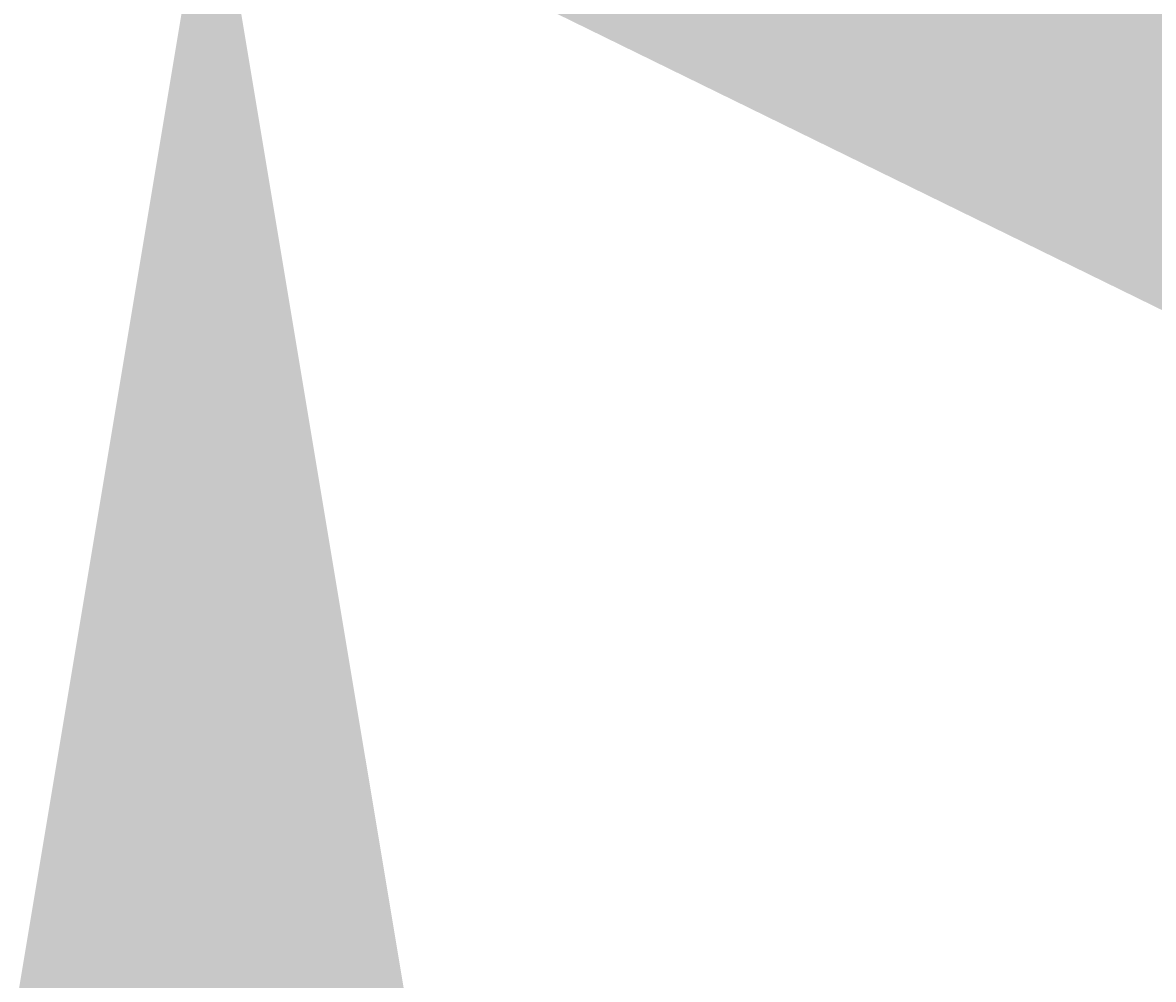
# Model space of a CAD drawing. Units: millimetres. Extents: x -22994 to 29398, y -19990 to 20176.
# Tile 5 of 135: x -44 to 2052, y -1986 to -212. Entities that reach past the tile are written whole.
import ezdxf

# ---------------------------------------------------------------- set-up
doc = ezdxf.new("R2010")
doc.units = ezdxf.units.MM
doc.header["$MEASUREMENT"] = 0
doc.layers.add('M-DIMS', color=2, linetype='Continuous', lineweight=18)
doc.styles.get("Standard").update_dxf_attribs({"font": 'arial.ttf'})
doc.dimstyles.get("Standard").update_dxf_attribs({"dimtxt": 0.18, "dimasz": 10000, "dimexe": 0.18, "dimexo": 0.0625, "dimgap": 0.09, "dimtad": 0, "dimtih": 1, "dimtoh": 1, "dimdec": 0, "dimzin": 0, "dimdsep": 46, "dimtxsty": 'Standard', "dimcen": 0.09, "dimadec": 0, "dimazin": 0, "dimtfac": 1, "dimtdec": 0, "dimtofl": 0, "dimtmove": 0, "dimatfit": 3, "dimfxl": 1, "dimtolj": 1, "dimtzin": 0, "dimlwd": 30, "dimarcsym": 0})

# ---------------------------------------------------------------- blocks, each defined once
blk = doc.blocks.new('*D2')
at = {"layer": 'Defpoints', "color": 0, "transparency": 16777216}
for p in [(6.7, 10.3), (290.9, 10.3), (290.9, -5.1)]:
    blk.add_point(p, dxfattribs=at)
at = {"layer": 'M-DIMS', "color": 0, "lineweight": -2, "transparency": 16777216}
for p, q in [((6.7, 10.2), (6.7, -5.3)), ((290.9, 10.2), (290.9, -5.3))]:
    blk.add_line(p, q, dxfattribs=at)
at = {"layer": 'M-DIMS', "color": 0, "lineweight": 30, "transparency": 16777216}
for p, q in [((-9993.3, -5.1), (-19993.3, -5.1)), ((10290.9, -5.1), (20290.9, -5.1))]:
    blk.add_line(p, q, dxfattribs=at)
at = {"layer": 'M-DIMS', "color": 0, "transparency": 16777216}
for points in [[(-9993.3, 1661.6), (-9993.3, -1671.7), (6.7, -5.1)], [(10290.9, 1661.6), (10290.9, -1671.7), (290.9, -5.1)]]:
    blk.add_solid(points, dxfattribs=at)
at = {"layer": 'M-DIMS', "color": 0, "transparency": 16777216, "insert": (148.8, -5.1), "char_height": 0.18, "attachment_point": 5}
blk.add_mtext('\\A1;284.2', dxfattribs=at)
blk = doc.blocks.new('*D3')
at = {"layer": 'Defpoints', "color": 0, "transparency": 16777216}
for p in [(110.3, 204.2), (110.3, 176.4), (95.8, 128)]:
    blk.add_point(p, dxfattribs=at)
at = {"layer": 'M-DIMS', "color": 0, "lineweight": 30, "transparency": 16777216}
for p, q in [((-9904.2, 204.2), (-19904.2, 204.2)), ((10110.3, 204.2), (20110.3, 204.2))]:
    blk.add_line(p, q, dxfattribs=at)
at = {"layer": 'M-DIMS', "color": 0, "lineweight": -2, "transparency": 16777216}
for p, q in [((95.8, 128), (95.8, 204.3)), ((110.3, 176.4), (110.3, 204.3))]:
    blk.add_line(p, q, dxfattribs=at)
at = {"layer": 'M-DIMS', "color": 0, "transparency": 16777216}
for points in [[(-9904.2, 1870.8), (-9904.2, -1462.5), (95.8, 204.2)], [(10110.3, 1870.8), (10110.3, -1462.5), (110.3, 204.2)]]:
    blk.add_solid(points, dxfattribs=at)
at = {"layer": 'M-DIMS', "color": 0, "transparency": 16777216, "insert": (103, 204.2), "char_height": 0.18, "attachment_point": 5}
blk.add_mtext('\\A1;14.432', dxfattribs=at)
blk = doc.blocks.new('*D4')
at = {"layer": 'Defpoints', "color": 0, "transparency": 16777216}
for p in [(116.3, 204.2), (110.3, 176.4), (116.3, 176.4)]:
    blk.add_point(p, dxfattribs=at)
at = {"layer": 'M-DIMS', "color": 0, "lineweight": 30, "transparency": 16777216}
for p, q in [((-9889.7, 204.2), (-19889.7, 204.2)), ((10116.3, 204.2), (20116.3, 204.2))]:
    blk.add_line(p, q, dxfattribs=at)
at = {"layer": 'M-DIMS', "color": 0, "lineweight": -2, "transparency": 16777216}
for p, q in [((110.3, 176.4), (110.3, 204.3)), ((116.3, 176.4), (116.3, 204.3))]:
    blk.add_line(p, q, dxfattribs=at)
at = {"layer": 'M-DIMS', "color": 0, "transparency": 16777216}
for points in [[(-9889.7, 1870.8), (-9889.7, -1462.5), (110.3, 204.2)], [(10116.3, 1870.8), (10116.3, -1462.5), (116.3, 204.2)]]:
    blk.add_solid(points, dxfattribs=at)
at = {"layer": 'M-DIMS', "color": 0, "transparency": 16777216, "insert": (113.3, 204.2), "char_height": 0.18, "attachment_point": 5}
blk.add_mtext('\\A1;6', dxfattribs=at)
blk = doc.blocks.new('*D5')
at = {"layer": 'Defpoints', "color": 0, "transparency": 16777216}
for p in [(181.3, 204.2), (116.3, 176.4), (181.3, 176.4)]:
    blk.add_point(p, dxfattribs=at)
at = {"layer": 'M-DIMS', "color": 0, "lineweight": 30, "transparency": 16777216}
for p, q in [((-9883.7, 204.2), (-19883.7, 204.2)), ((10181.3, 204.2), (20181.3, 204.2))]:
    blk.add_line(p, q, dxfattribs=at)
at = {"layer": 'M-DIMS', "color": 0, "lineweight": -2, "transparency": 16777216}
for p, q in [((116.3, 176.4), (116.3, 204.3)), ((181.3, 176.4), (181.3, 204.3))]:
    blk.add_line(p, q, dxfattribs=at)
at = {"layer": 'M-DIMS', "color": 0, "transparency": 16777216}
for points in [[(-9883.7, 1870.8), (-9883.7, -1462.5), (116.3, 204.2)], [(10181.3, 1870.8), (10181.3, -1462.5), (181.3, 204.2)]]:
    blk.add_solid(points, dxfattribs=at)
at = {"layer": 'M-DIMS', "color": 0, "transparency": 16777216, "insert": (148.8, 204.2), "char_height": 0.18, "attachment_point": 5}
blk.add_mtext('\\A1;65', dxfattribs=at)
blk = doc.blocks.new('*D6')
at = {"layer": 'Defpoints', "color": 0, "transparency": 16777216}
for p in [(187.3, 204.2), (181.3, 176.4), (187.3, 176.4)]:
    blk.add_point(p, dxfattribs=at)
at = {"layer": 'M-DIMS', "color": 0, "lineweight": 30, "transparency": 16777216}
for p, q in [((-9818.7, 204.2), (-19818.7, 204.2)), ((10187.3, 204.2), (20187.3, 204.2))]:
    blk.add_line(p, q, dxfattribs=at)
at = {"layer": 'M-DIMS', "color": 0, "lineweight": -2, "transparency": 16777216}
for p, q in [((181.3, 176.4), (181.3, 204.3)), ((187.3, 176.4), (187.3, 204.3))]:
    blk.add_line(p, q, dxfattribs=at)
at = {"layer": 'M-DIMS', "color": 0, "transparency": 16777216}
for points in [[(-9818.7, 1870.8), (-9818.7, -1462.5), (181.3, 204.2)], [(10187.3, 1870.8), (10187.3, -1462.5), (187.3, 204.2)]]:
    blk.add_solid(points, dxfattribs=at)
at = {"layer": 'M-DIMS', "color": 0, "transparency": 16777216, "insert": (184.3, 204.2), "char_height": 0.18, "attachment_point": 5}
blk.add_mtext('\\A1;6', dxfattribs=at)
blk = doc.blocks.new('*D7')
at = {"layer": 'Defpoints', "color": 0, "transparency": 16777216}
for p in [(201.7, 204.2), (187.3, 176.4), (201.7, 128)]:
    blk.add_point(p, dxfattribs=at)
at = {"layer": 'M-DIMS', "color": 0, "lineweight": 30, "transparency": 16777216}
for p, q in [((-9812.7, 204.2), (-19812.7, 204.2)), ((10201.7, 204.2), (20201.7, 204.2))]:
    blk.add_line(p, q, dxfattribs=at)
at = {"layer": 'M-DIMS', "color": 0, "lineweight": -2, "transparency": 16777216}
for p, q in [((187.3, 176.4), (187.3, 204.3)), ((201.7, 128), (201.7, 204.3))]:
    blk.add_line(p, q, dxfattribs=at)
at = {"layer": 'M-DIMS', "color": 0, "transparency": 16777216}
for points in [[(-9812.7, 1870.8), (-9812.7, -1462.5), (187.3, 204.2)], [(10201.7, 1870.8), (10201.7, -1462.5), (201.7, 204.2)]]:
    blk.add_solid(points, dxfattribs=at)
at = {"layer": 'M-DIMS', "color": 0, "transparency": 16777216, "insert": (194.5, 204.2), "char_height": 0.18, "attachment_point": 5}
blk.add_mtext('\\A1;14.432', dxfattribs=at)
blk = doc.blocks.new('*D8')
at = {"layer": 'Defpoints', "color": 0, "transparency": 16777216}
for p in [(227.6, 204.2), (227.6, 146.7), (201.7, 128)]:
    blk.add_point(p, dxfattribs=at)
at = {"layer": 'M-DIMS', "color": 0, "lineweight": 30, "transparency": 16777216}
for p, q in [((-9798.3, 204.2), (-19798.3, 204.2)), ((10227.6, 204.2), (20227.6, 204.2))]:
    blk.add_line(p, q, dxfattribs=at)
at = {"layer": 'M-DIMS', "color": 0, "lineweight": -2, "transparency": 16777216}
for p, q in [((201.7, 128), (201.7, 204.3)), ((227.6, 146.8), (227.6, 204.3))]:
    blk.add_line(p, q, dxfattribs=at)
at = {"layer": 'M-DIMS', "color": 0, "transparency": 16777216}
for points in [[(-9798.3, 1870.8), (-9798.3, -1462.5), (201.7, 204.2)], [(10227.6, 1870.8), (10227.6, -1462.5), (227.6, 204.2)]]:
    blk.add_solid(points, dxfattribs=at)
at = {"layer": 'M-DIMS', "color": 0, "transparency": 16777216, "insert": (214.7, 204.2), "char_height": 0.18, "attachment_point": 5}
blk.add_mtext('\\A1;25.95', dxfattribs=at)
blk = doc.blocks.new('*D9')
at = {"layer": 'Defpoints', "color": 0, "transparency": 16777216}
for p in [(187.3, 176.4), (306.2, 176.4), (290.9, 10.3)]:
    blk.add_point(p, dxfattribs=at)
at = {"layer": 'M-DIMS', "color": 0, "lineweight": 30, "transparency": 16777216}
for p, q in [((306.2, 10176.4), (306.2, 20176.4)), ((306.2, -9989.7), (306.2, -19989.7))]:
    blk.add_line(p, q, dxfattribs=at)
at = {"layer": 'M-DIMS', "color": 0, "lineweight": -2, "transparency": 16777216}
for p, q in [((187.3, 176.4), (306.4, 176.4)), ((290.9, 10.3), (306.4, 10.3))]:
    blk.add_line(p, q, dxfattribs=at)
at = {"layer": 'M-DIMS', "color": 0, "transparency": 16777216}
for points in [[(-1360.5, 10176.4), (1972.9, 10176.4), (306.2, 176.4)], [(-1360.5, -9989.7), (1972.9, -9989.7), (306.2, 10.3)]]:
    blk.add_solid(points, dxfattribs=at)
at = {"layer": 'M-DIMS', "color": 0, "transparency": 16777216, "insert": (306.2, 93.3), "char_height": 0.18, "attachment_point": 5}
blk.add_mtext('\\A1;166.1', dxfattribs=at)
blk = doc.blocks.new('*D10')
at = {"layer": 'Defpoints', "color": 0, "transparency": 16777216}
for p in [(125.6, 136.1), (133.3, 136.1), (133.3, -5.1)]:
    blk.add_point(p, dxfattribs=at)
at = {"layer": 'M-DIMS', "color": 0, "lineweight": -2, "transparency": 16777216}
for p, q in [((125.6, 136), (125.6, -5.3)), ((133.3, 136), (133.3, -5.3))]:
    blk.add_line(p, q, dxfattribs=at)
at = {"layer": 'M-DIMS', "color": 0, "lineweight": 30, "transparency": 16777216}
for p, q in [((-9874.4, -5.1), (-19874.4, -5.1)), ((10133.3, -5.1), (20133.3, -5.1))]:
    blk.add_line(p, q, dxfattribs=at)
at = {"layer": 'M-DIMS', "color": 0, "transparency": 16777216}
for points in [[(-9874.4, 1661.6), (-9874.4, -1671.7), (125.6, -5.1)], [(10133.3, 1661.6), (10133.3, -1671.7), (133.3, -5.1)]]:
    blk.add_solid(points, dxfattribs=at)
at = {"layer": 'M-DIMS', "color": 0, "transparency": 16777216, "insert": (129.5, -5.1), "char_height": 0.18, "attachment_point": 5}
blk.add_mtext('\\A1;7.696', dxfattribs=at)
blk = doc.blocks.new('*D11')
at = {"layer": 'Defpoints', "color": 0, "transparency": 16777216}
for p in [(133.3, 136.1), (135.6, 136.1), (135.6, -5.1)]:
    blk.add_point(p, dxfattribs=at)
at = {"layer": 'M-DIMS', "color": 0, "lineweight": -2, "transparency": 16777216}
for p, q in [((133.3, 136), (133.3, -5.3)), ((135.6, 136), (135.6, -5.3))]:
    blk.add_line(p, q, dxfattribs=at)
at = {"layer": 'M-DIMS', "color": 0, "lineweight": 30, "transparency": 16777216}
for p, q in [((-9866.7, -5.1), (-19866.7, -5.1)), ((10135.6, -5.1), (20135.6, -5.1))]:
    blk.add_line(p, q, dxfattribs=at)
at = {"layer": 'M-DIMS', "color": 0, "transparency": 16777216}
for points in [[(-9866.7, 1661.6), (-9866.7, -1671.7), (133.3, -5.1)], [(10135.6, 1661.6), (10135.6, -1671.7), (135.6, -5.1)]]:
    blk.add_solid(points, dxfattribs=at)
at = {"layer": 'M-DIMS', "color": 0, "transparency": 16777216, "insert": (134.5, -5.1), "char_height": 0.18, "attachment_point": 5}
blk.add_mtext('\\A1;2.304', dxfattribs=at)
blk = doc.blocks.new('*D12')
at = {"layer": 'Defpoints', "color": 0, "transparency": 16777216}
for p in [(135.6, 136.1), (145.6, 136.1), (145.6, -5.1)]:
    blk.add_point(p, dxfattribs=at)
at = {"layer": 'M-DIMS', "color": 0, "lineweight": -2, "transparency": 16777216}
for p, q in [((135.6, 136), (135.6, -5.3)), ((145.6, 136), (145.6, -5.3))]:
    blk.add_line(p, q, dxfattribs=at)
at = {"layer": 'M-DIMS', "color": 0, "lineweight": 30, "transparency": 16777216}
for p, q in [((-9864.4, -5.1), (-19864.4, -5.1)), ((10145.6, -5.1), (20145.6, -5.1))]:
    blk.add_line(p, q, dxfattribs=at)
at = {"layer": 'M-DIMS', "color": 0, "transparency": 16777216}
for points in [[(-9864.4, 1661.6), (-9864.4, -1671.7), (135.6, -5.1)], [(10145.6, 1661.6), (10145.6, -1671.7), (145.6, -5.1)]]:
    blk.add_solid(points, dxfattribs=at)
at = {"layer": 'M-DIMS', "color": 0, "transparency": 16777216, "insert": (140.6, -5.1), "char_height": 0.18, "attachment_point": 5}
blk.add_mtext('\\A1;10', dxfattribs=at)
blk = doc.blocks.new('*D13')
at = {"layer": 'Defpoints', "color": 0, "transparency": 16777216}
for p in [(145.6, 136.1), (155.6, 136.1), (155.6, -5.1)]:
    blk.add_point(p, dxfattribs=at)
at = {"layer": 'M-DIMS', "color": 0, "lineweight": -2, "transparency": 16777216}
for p, q in [((145.6, 136), (145.6, -5.3)), ((155.6, 136), (155.6, -5.3))]:
    blk.add_line(p, q, dxfattribs=at)
at = {"layer": 'M-DIMS', "color": 0, "lineweight": 30, "transparency": 16777216}
for p, q in [((-9854.4, -5.1), (-19854.4, -5.1)), ((10155.6, -5.1), (20155.6, -5.1))]:
    blk.add_line(p, q, dxfattribs=at)
at = {"layer": 'M-DIMS', "color": 0, "transparency": 16777216}
for points in [[(-9854.4, 1661.6), (-9854.4, -1671.7), (145.6, -5.1)], [(10155.6, 1661.6), (10155.6, -1671.7), (155.6, -5.1)]]:
    blk.add_solid(points, dxfattribs=at)
at = {"layer": 'M-DIMS', "color": 0, "transparency": 16777216, "insert": (150.6, -5.1), "char_height": 0.18, "attachment_point": 5}
blk.add_mtext('\\A1;10', dxfattribs=at)
blk = doc.blocks.new('*D14')
at = {"layer": 'Defpoints', "color": 0, "transparency": 16777216}
for p in [(155.6, 136.1), (165.6, 136.1), (165.6, -5.1)]:
    blk.add_point(p, dxfattribs=at)
at = {"layer": 'M-DIMS', "color": 0, "lineweight": -2, "transparency": 16777216}
for p, q in [((155.6, 136), (155.6, -5.3)), ((165.6, 136), (165.6, -5.3))]:
    blk.add_line(p, q, dxfattribs=at)
at = {"layer": 'M-DIMS', "color": 0, "lineweight": 30, "transparency": 16777216}
for p, q in [((-9844.4, -5.1), (-19844.4, -5.1)), ((10165.6, -5.1), (20165.6, -5.1))]:
    blk.add_line(p, q, dxfattribs=at)
at = {"layer": 'M-DIMS', "color": 0, "transparency": 16777216}
for points in [[(-9844.4, 1661.6), (-9844.4, -1671.7), (155.6, -5.1)], [(10165.6, 1661.6), (10165.6, -1671.7), (165.6, -5.1)]]:
    blk.add_solid(points, dxfattribs=at)
at = {"layer": 'M-DIMS', "color": 0, "transparency": 16777216, "insert": (160.6, -5.1), "char_height": 0.18, "attachment_point": 5}
blk.add_mtext('\\A1;10', dxfattribs=at)
blk = doc.blocks.new('*D15')
at = {"layer": 'Defpoints', "color": 0, "transparency": 16777216}
for p in [(173.3, 154.8), (173.3, 136.1), (306.2, 136.1)]:
    blk.add_point(p, dxfattribs=at)
at = {"layer": 'M-DIMS', "color": 0, "lineweight": 30, "transparency": 16777216}
for p, q in [((306.2, 10154.8), (306.2, 20154.8)), ((306.2, -9863.9), (306.2, -19863.9))]:
    blk.add_line(p, q, dxfattribs=at)
at = {"layer": 'M-DIMS', "color": 0, "lineweight": -2, "transparency": 16777216}
for p, q in [((173.4, 154.8), (306.4, 154.8)), ((173.4, 136.1), (306.4, 136.1))]:
    blk.add_line(p, q, dxfattribs=at)
at = {"layer": 'M-DIMS', "color": 0, "transparency": 16777216}
for points in [[(-1360.5, 10154.8), (1972.9, 10154.8), (306.2, 154.8)], [(-1360.5, -9863.9), (1972.9, -9863.9), (306.2, 136.1)]]:
    blk.add_solid(points, dxfattribs=at)
at = {"layer": 'M-DIMS', "color": 0, "transparency": 16777216, "insert": (306.2, 145.4), "char_height": 0.18, "attachment_point": 5}
blk.add_mtext('\\A1;18.717', dxfattribs=at)
blk = doc.blocks.new('*D16')
at = {"layer": 'Defpoints', "color": 0, "transparency": 16777216}
for p in [(120.2, 204.2), (110.5, 48), (120.2, 48)]:
    blk.add_point(p, dxfattribs=at)
at = {"layer": 'M-DIMS', "color": 0, "lineweight": 30, "transparency": 16777216}
for p, q in [((-9889.5, 204.2), (-19889.5, 204.2)), ((10120.2, 204.2), (20120.2, 204.2))]:
    blk.add_line(p, q, dxfattribs=at)
at = {"layer": 'M-DIMS', "color": 0, "lineweight": -2, "transparency": 16777216}
for p, q in [((110.5, 48.1), (110.5, 204.3)), ((120.2, 48.1), (120.2, 204.3))]:
    blk.add_line(p, q, dxfattribs=at)
at = {"layer": 'M-DIMS', "color": 0, "transparency": 16777216}
for points in [[(-9889.5, 1870.8), (-9889.5, -1462.5), (110.5, 204.2)], [(10120.2, 1870.8), (10120.2, -1462.5), (120.2, 204.2)]]:
    blk.add_solid(points, dxfattribs=at)
at = {"layer": 'M-DIMS', "color": 0, "transparency": 16777216, "insert": (115.3, 204.2), "char_height": 0.18, "attachment_point": 5}
blk.add_mtext('\\A1;9.704', dxfattribs=at)
blk = doc.blocks.new('*D17')
at = {"layer": 'Defpoints', "color": 0, "transparency": 16777216}
for p in [(126.2, 204.2), (120.2, 48), (126.2, 48)]:
    blk.add_point(p, dxfattribs=at)
at = {"layer": 'M-DIMS', "color": 0, "lineweight": 30, "transparency": 16777216}
for p, q in [((-9879.8, 204.2), (-19879.8, 204.2)), ((10126.2, 204.2), (20126.2, 204.2))]:
    blk.add_line(p, q, dxfattribs=at)
at = {"layer": 'M-DIMS', "color": 0, "lineweight": -2, "transparency": 16777216}
for p, q in [((120.2, 48.1), (120.2, 204.3)), ((126.2, 48.1), (126.2, 204.3))]:
    blk.add_line(p, q, dxfattribs=at)
at = {"layer": 'M-DIMS', "color": 0, "transparency": 16777216}
for points in [[(-9879.8, 1870.8), (-9879.8, -1462.5), (120.2, 204.2)], [(10126.2, 1870.8), (10126.2, -1462.5), (126.2, 204.2)]]:
    blk.add_solid(points, dxfattribs=at)
at = {"layer": 'M-DIMS', "color": 0, "transparency": 16777216, "insert": (123.2, 204.2), "char_height": 0.18, "attachment_point": 5}
blk.add_mtext('\\A1;6', dxfattribs=at)
blk = doc.blocks.new('*D18')
at = {"layer": 'Defpoints', "color": 0, "transparency": 16777216}
for p in [(132.2, 204.2), (126.2, 48), (132.2, 48)]:
    blk.add_point(p, dxfattribs=at)
at = {"layer": 'M-DIMS', "color": 0, "lineweight": 30, "transparency": 16777216}
for p, q in [((-9873.8, 204.2), (-19873.8, 204.2)), ((10132.2, 204.2), (20132.2, 204.2))]:
    blk.add_line(p, q, dxfattribs=at)
at = {"layer": 'M-DIMS', "color": 0, "lineweight": -2, "transparency": 16777216}
for p, q in [((126.2, 48.1), (126.2, 204.3)), ((132.2, 48.1), (132.2, 204.3))]:
    blk.add_line(p, q, dxfattribs=at)
at = {"layer": 'M-DIMS', "color": 0, "transparency": 16777216}
for points in [[(-9873.8, 1870.8), (-9873.8, -1462.5), (126.2, 204.2)], [(10132.2, 1870.8), (10132.2, -1462.5), (132.2, 204.2)]]:
    blk.add_solid(points, dxfattribs=at)
at = {"layer": 'M-DIMS', "color": 0, "transparency": 16777216, "insert": (129.2, 204.2), "char_height": 0.18, "attachment_point": 5}
blk.add_mtext('\\A1;6', dxfattribs=at)
blk = doc.blocks.new('*D19')
at = {"layer": 'Defpoints', "color": 0, "transparency": 16777216}
for p in [(138.2, 204.2), (132.2, 48), (138.2, 48)]:
    blk.add_point(p, dxfattribs=at)
at = {"layer": 'M-DIMS', "color": 0, "lineweight": 30, "transparency": 16777216}
for p, q in [((-9867.8, 204.2), (-19867.8, 204.2)), ((10138.2, 204.2), (20138.2, 204.2))]:
    blk.add_line(p, q, dxfattribs=at)
at = {"layer": 'M-DIMS', "color": 0, "lineweight": -2, "transparency": 16777216}
for p, q in [((132.2, 48.1), (132.2, 204.3)), ((138.2, 48.1), (138.2, 204.3))]:
    blk.add_line(p, q, dxfattribs=at)
at = {"layer": 'M-DIMS', "color": 0, "transparency": 16777216}
for points in [[(-9867.8, 1870.8), (-9867.8, -1462.5), (132.2, 204.2)], [(10138.2, 1870.8), (10138.2, -1462.5), (138.2, 204.2)]]:
    blk.add_solid(points, dxfattribs=at)
at = {"layer": 'M-DIMS', "color": 0, "transparency": 16777216, "insert": (135.2, 204.2), "char_height": 0.18, "attachment_point": 5}
blk.add_mtext('\\A1;6', dxfattribs=at)
blk = doc.blocks.new('*D20')
at = {"layer": 'Defpoints', "color": 0, "transparency": 16777216}
for p in [(144.2, 204.2), (138.2, 48), (144.2, 48)]:
    blk.add_point(p, dxfattribs=at)
at = {"layer": 'M-DIMS', "color": 0, "lineweight": 30, "transparency": 16777216}
for p, q in [((-9861.8, 204.2), (-19861.8, 204.2)), ((10144.2, 204.2), (20144.2, 204.2))]:
    blk.add_line(p, q, dxfattribs=at)
at = {"layer": 'M-DIMS', "color": 0, "lineweight": -2, "transparency": 16777216}
for p, q in [((138.2, 48.1), (138.2, 204.3)), ((144.2, 48.1), (144.2, 204.3))]:
    blk.add_line(p, q, dxfattribs=at)
at = {"layer": 'M-DIMS', "color": 0, "transparency": 16777216}
for points in [[(-9861.8, 1870.8), (-9861.8, -1462.5), (138.2, 204.2)], [(10144.2, 1870.8), (10144.2, -1462.5), (144.2, 204.2)]]:
    blk.add_solid(points, dxfattribs=at)
at = {"layer": 'M-DIMS', "color": 0, "transparency": 16777216, "insert": (141.2, 204.2), "char_height": 0.18, "attachment_point": 5}
blk.add_mtext('\\A1;6', dxfattribs=at)
blk = doc.blocks.new('*D21')
at = {"layer": 'Defpoints', "color": 0, "transparency": 16777216}
for p in [(149.1, 204.2), (144.2, 48), (149.1, 48)]:
    blk.add_point(p, dxfattribs=at)
at = {"layer": 'M-DIMS', "color": 0, "lineweight": 30, "transparency": 16777216}
for p, q in [((-9855.8, 204.2), (-19855.8, 204.2)), ((10149.1, 204.2), (20149.1, 204.2))]:
    blk.add_line(p, q, dxfattribs=at)
at = {"layer": 'M-DIMS', "color": 0, "lineweight": -2, "transparency": 16777216}
for p, q in [((144.2, 48.1), (144.2, 204.3)), ((149.1, 48.1), (149.1, 204.3))]:
    blk.add_line(p, q, dxfattribs=at)
at = {"layer": 'M-DIMS', "color": 0, "transparency": 16777216}
for points in [[(-9855.8, 1870.8), (-9855.8, -1462.5), (144.2, 204.2)], [(10149.1, 1870.8), (10149.1, -1462.5), (149.1, 204.2)]]:
    blk.add_solid(points, dxfattribs=at)
at = {"layer": 'M-DIMS', "color": 0, "transparency": 16777216, "insert": (146.6, 204.2), "char_height": 0.18, "attachment_point": 5}
blk.add_mtext('\\A1;4.945', dxfattribs=at)
blk = doc.blocks.new('*D22')
at = {"layer": 'Defpoints', "color": 0, "transparency": 16777216}
for p in [(149.1, 31), (155.1, 31), (155.1, -5.1)]:
    blk.add_point(p, dxfattribs=at)
at = {"layer": 'M-DIMS', "color": 0, "lineweight": -2, "transparency": 16777216}
for p, q in [((149.1, 30.9), (149.1, -5.3)), ((155.1, 30.9), (155.1, -5.3))]:
    blk.add_line(p, q, dxfattribs=at)
at = {"layer": 'M-DIMS', "color": 0, "lineweight": 30, "transparency": 16777216}
for p, q in [((-9850.9, -5.1), (-19850.9, -5.1)), ((10155.1, -5.1), (20155.1, -5.1))]:
    blk.add_line(p, q, dxfattribs=at)
at = {"layer": 'M-DIMS', "color": 0, "transparency": 16777216}
for points in [[(-9850.9, 1661.6), (-9850.9, -1671.7), (149.1, -5.1)], [(10155.1, 1661.6), (10155.1, -1671.7), (155.1, -5.1)]]:
    blk.add_solid(points, dxfattribs=at)
at = {"layer": 'M-DIMS', "color": 0, "transparency": 16777216, "insert": (152.1, -5.1), "char_height": 0.18, "attachment_point": 5}
blk.add_mtext('\\A1;6', dxfattribs=at)
blk = doc.blocks.new('*D23')
at = {"layer": 'Defpoints', "color": 0, "transparency": 16777216}
for p in [(155.1, 31), (161.1, 31), (161.1, -5.1)]:
    blk.add_point(p, dxfattribs=at)
at = {"layer": 'M-DIMS', "color": 0, "lineweight": -2, "transparency": 16777216}
for p, q in [((155.1, 30.9), (155.1, -5.3)), ((161.1, 30.9), (161.1, -5.3))]:
    blk.add_line(p, q, dxfattribs=at)
at = {"layer": 'M-DIMS', "color": 0, "lineweight": 30, "transparency": 16777216}
for p, q in [((-9844.9, -5.1), (-19844.9, -5.1)), ((10161.1, -5.1), (20161.1, -5.1))]:
    blk.add_line(p, q, dxfattribs=at)
at = {"layer": 'M-DIMS', "color": 0, "transparency": 16777216}
for points in [[(-9844.9, 1661.6), (-9844.9, -1671.7), (155.1, -5.1)], [(10161.1, 1661.6), (10161.1, -1671.7), (161.1, -5.1)]]:
    blk.add_solid(points, dxfattribs=at)
at = {"layer": 'M-DIMS', "color": 0, "transparency": 16777216, "insert": (158.1, -5.1), "char_height": 0.18, "attachment_point": 5}
blk.add_mtext('\\A1;6', dxfattribs=at)
blk = doc.blocks.new('*D24')
at = {"layer": 'Defpoints', "color": 0, "transparency": 16777216}
for p in [(161.1, 31), (166.4, 31), (166.4, -5.1)]:
    blk.add_point(p, dxfattribs=at)
at = {"layer": 'M-DIMS', "color": 0, "lineweight": -2, "transparency": 16777216}
for p, q in [((161.1, 30.9), (161.1, -5.3)), ((166.4, 30.9), (166.4, -5.3))]:
    blk.add_line(p, q, dxfattribs=at)
at = {"layer": 'M-DIMS', "color": 0, "lineweight": 30, "transparency": 16777216}
for p, q in [((-9838.9, -5.1), (-19838.9, -5.1)), ((10166.4, -5.1), (20166.4, -5.1))]:
    blk.add_line(p, q, dxfattribs=at)
at = {"layer": 'M-DIMS', "color": 0, "transparency": 16777216}
for points in [[(-9838.9, 1661.6), (-9838.9, -1671.7), (161.1, -5.1)], [(10166.4, 1661.6), (10166.4, -1671.7), (166.4, -5.1)]]:
    blk.add_solid(points, dxfattribs=at)
at = {"layer": 'M-DIMS', "color": 0, "transparency": 16777216, "insert": (163.8, -5.1), "char_height": 0.18, "attachment_point": 5}
blk.add_mtext('\\A1;5.323', dxfattribs=at)
blk = doc.blocks.new('*D25')
at = {"layer": 'Defpoints', "color": 0, "transparency": 16777216}
for p in [(166.4, 31), (172.4, 31), (172.4, -5.1)]:
    blk.add_point(p, dxfattribs=at)
at = {"layer": 'M-DIMS', "color": 0, "lineweight": -2, "transparency": 16777216}
for p, q in [((166.4, 30.9), (166.4, -5.3)), ((172.4, 30.9), (172.4, -5.3))]:
    blk.add_line(p, q, dxfattribs=at)
at = {"layer": 'M-DIMS', "color": 0, "lineweight": 30, "transparency": 16777216}
for p, q in [((-9833.6, -5.1), (-19833.6, -5.1)), ((10172.4, -5.1), (20172.4, -5.1))]:
    blk.add_line(p, q, dxfattribs=at)
at = {"layer": 'M-DIMS', "color": 0, "transparency": 16777216}
for points in [[(-9833.6, 1661.6), (-9833.6, -1671.7), (166.4, -5.1)], [(10172.4, 1661.6), (10172.4, -1671.7), (172.4, -5.1)]]:
    blk.add_solid(points, dxfattribs=at)
at = {"layer": 'M-DIMS', "color": 0, "transparency": 16777216, "insert": (169.4, -5.1), "char_height": 0.18, "attachment_point": 5}
blk.add_mtext('\\A1;6', dxfattribs=at)
blk = doc.blocks.new('*D26')
at = {"layer": 'Defpoints', "color": 0, "transparency": 16777216}
for p in [(172.4, 31), (178.4, 31), (178.4, -5.1)]:
    blk.add_point(p, dxfattribs=at)
at = {"layer": 'M-DIMS', "color": 0, "lineweight": -2, "transparency": 16777216}
for p, q in [((172.4, 30.9), (172.4, -5.3)), ((178.4, 30.9), (178.4, -5.3))]:
    blk.add_line(p, q, dxfattribs=at)
at = {"layer": 'M-DIMS', "color": 0, "lineweight": 30, "transparency": 16777216}
for p, q in [((-9827.6, -5.1), (-19827.6, -5.1)), ((10178.4, -5.1), (20178.4, -5.1))]:
    blk.add_line(p, q, dxfattribs=at)
at = {"layer": 'M-DIMS', "color": 0, "transparency": 16777216}
for points in [[(-9827.6, 1661.6), (-9827.6, -1671.7), (172.4, -5.1)], [(10178.4, 1661.6), (10178.4, -1671.7), (178.4, -5.1)]]:
    blk.add_solid(points, dxfattribs=at)
at = {"layer": 'M-DIMS', "color": 0, "transparency": 16777216, "insert": (175.4, -5.1), "char_height": 0.18, "attachment_point": 5}
blk.add_mtext('\\A1;6', dxfattribs=at)
blk = doc.blocks.new('*D27')
at = {"layer": 'Defpoints', "color": 0, "transparency": 16777216}
for p in [(178.4, 31), (188.1, 31), (188.1, -5.1)]:
    blk.add_point(p, dxfattribs=at)
at = {"layer": 'M-DIMS', "color": 0, "lineweight": -2, "transparency": 16777216}
for p, q in [((178.4, 30.9), (178.4, -5.3)), ((188.1, 30.9), (188.1, -5.3))]:
    blk.add_line(p, q, dxfattribs=at)
at = {"layer": 'M-DIMS', "color": 0, "lineweight": 30, "transparency": 16777216}
for p, q in [((-9821.6, -5.1), (-19821.6, -5.1)), ((10188.1, -5.1), (20188.1, -5.1))]:
    blk.add_line(p, q, dxfattribs=at)
at = {"layer": 'M-DIMS', "color": 0, "transparency": 16777216}
for points in [[(-9821.6, 1661.6), (-9821.6, -1671.7), (178.4, -5.1)], [(10188.1, 1661.6), (10188.1, -1671.7), (188.1, -5.1)]]:
    blk.add_solid(points, dxfattribs=at)
at = {"layer": 'M-DIMS', "color": 0, "transparency": 16777216, "insert": (183.3, -5.1), "char_height": 0.18, "attachment_point": 5}
blk.add_mtext('\\A1;9.679', dxfattribs=at)
blk = doc.blocks.new('*D28')
at = {"layer": 'Defpoints', "color": 0, "transparency": 16777216}
for p in [(188.1, 48), (306.2, 48), (188.1, 31)]:
    blk.add_point(p, dxfattribs=at)
at = {"layer": 'M-DIMS', "color": 0, "lineweight": 30, "transparency": 16777216}
for p, q in [((306.2, 10048), (306.2, 20048)), ((306.2, -9969), (306.2, -19969))]:
    blk.add_line(p, q, dxfattribs=at)
at = {"layer": 'M-DIMS', "color": 0, "lineweight": -2, "transparency": 16777216}
for p, q in [((188.2, 48), (306.4, 48)), ((188.2, 31), (306.4, 31))]:
    blk.add_line(p, q, dxfattribs=at)
at = {"layer": 'M-DIMS', "color": 0, "transparency": 16777216}
for points in [[(-1360.5, 10048), (1972.9, 10048), (306.2, 48)], [(-1360.5, -9969), (1972.9, -9969), (306.2, 31)]]:
    blk.add_solid(points, dxfattribs=at)
at = {"layer": 'M-DIMS', "color": 0, "transparency": 16777216, "insert": (306.2, 39.5), "char_height": 0.18, "attachment_point": 5}
blk.add_mtext('\\A1;17.045', dxfattribs=at)
blk = doc.blocks.new('*D29')
at = {"layer": 'Defpoints', "color": 0, "transparency": 16777216}
for p in [(36.8, 80), (64, 80)]:
    blk.add_point(p, dxfattribs=at)
at = {"layer": 'M-DIMS', "color": 0, "lineweight": -2, "transparency": 16777216}
for p, q in [((50.3, 80), (50.5, 80)), ((50.4, 80), (50.4, 80.1))]:
    blk.add_line(p, q, dxfattribs=at)
at = {"layer": 'M-DIMS', "color": 0, "lineweight": 30, "transparency": 16777216}
blk.add_line((20064, 80), (10064, 80), dxfattribs=at)
at = {"layer": 'M-DIMS', "color": 0, "transparency": 16777216}
blk.add_solid([(10064, 1746.7), (10064, -1586.6), (64, 80)], dxfattribs=at)
at = {"layer": 'M-DIMS', "color": 0, "transparency": 16777216, "insert": (20064.5, 80), "char_height": 0.18, "attachment_point": 5}
blk.add_mtext('\\A1;∅27.23', dxfattribs=at)
blk = doc.blocks.new('*D30')
at = {"layer": 'Defpoints', "color": 0, "transparency": 16777216}
for p in [(216.3, 146.7), (239, 146.7)]:
    blk.add_point(p, dxfattribs=at)
at = {"layer": 'M-DIMS', "color": 0, "lineweight": -2, "transparency": 16777216}
for p, q in [((227.6, 146.6), (227.6, 146.8)), ((227.6, 146.7), (227.7, 146.7))]:
    blk.add_line(p, q, dxfattribs=at)
at = {"layer": 'M-DIMS', "color": 0, "lineweight": 30, "transparency": 16777216}
blk.add_line((20239, 147.5), (10239, 147.1), dxfattribs=at)
at = {"layer": 'M-DIMS', "color": 0, "transparency": 16777216}
blk.add_solid([(10238.9, 1813.8), (10239, -1519.6), (239, 146.7)], dxfattribs=at)
at = {"layer": 'M-DIMS', "color": 0, "transparency": 16777216, "insert": (20239.5, 147.5), "char_height": 0.18, "attachment_point": 5}
blk.add_mtext('\\A1;∅22.667', dxfattribs=at)
blk = doc.blocks.new('*D31')
at = {"layer": 'Defpoints', "color": 0, "transparency": 16777216}
for p in [(223.2, 146.7), (232.1, 146.7)]:
    blk.add_point(p, dxfattribs=at)
at = {"layer": 'M-DIMS', "color": 0, "lineweight": -2, "transparency": 16777216}
for p, q in [((227.6, 146.6), (227.6, 146.8)), ((227.6, 146.7), (227.7, 146.7))]:
    blk.add_line(p, q, dxfattribs=at)
at = {"layer": 'M-DIMS', "color": 0, "lineweight": 30, "transparency": 16777216}
blk.add_line((20232.1, 148.7), (10232.1, 147.7), dxfattribs=at)
at = {"layer": 'M-DIMS', "color": 0, "transparency": 16777216}
blk.add_solid([(10232, 1814.4), (10232.3, -1519), (232.1, 146.7)], dxfattribs=at)
at = {"layer": 'M-DIMS', "color": 0, "transparency": 16777216, "insert": (20232.6, 148.7), "char_height": 0.18, "attachment_point": 5}
blk.add_mtext('\\A1;∅8.969', dxfattribs=at)
blk = doc.blocks.new('*D32')
at = {"layer": 'Defpoints', "color": 0, "transparency": 16777216}
for p in [(52.4, 113.1), (57.2, 118.6)]:
    blk.add_point(p, dxfattribs=at)
at = {"layer": 'M-DIMS', "color": 0, "lineweight": -2, "transparency": 16777216}
for p, q in [((57.1, 118.6), (57.3, 118.6)), ((57.2, 118.5), (57.2, 118.7))]:
    blk.add_line(p, q, dxfattribs=at)
at = {"layer": 'M-DIMS', "color": 0, "lineweight": 30, "transparency": 16777216}
for p, q in [((-12992.5, -15047), (-6470.1, -7467)), ((-22992.5, -15047), (-12992.5, -15047))]:
    blk.add_line(p, q, dxfattribs=at)
at = {"layer": 'M-DIMS', "color": 0, "transparency": 16777216}
blk.add_solid([(-7733.4, -6379.9), (-5206.7, -8554), (52.4, 113.1)], dxfattribs=at)
at = {"layer": 'M-DIMS', "color": 0, "transparency": 16777216, "insert": (-22993.2, -15047), "char_height": 0.18, "attachment_point": 5}
blk.add_mtext('\\A1;2X R7.284', dxfattribs=at)
blk = doc.blocks.new('*D33')
at = {"layer": 'Defpoints', "color": 0, "transparency": 16777216}
for p in [(229.6, 154.4), (233, 153.4)]:
    blk.add_point(p, dxfattribs=at)
at = {"layer": 'M-DIMS', "color": 0, "lineweight": -2, "transparency": 16777216}
for p, q in [((229.5, 154.4), (229.7, 154.4)), ((229.6, 154.3), (229.6, 154.5))]:
    blk.add_line(p, q, dxfattribs=at)
at = {"layer": 'M-DIMS', "color": 0, "lineweight": 30, "transparency": 16777216}
for p, q in [((19396.3, -5570.8), (9814.7, -2708.7)), ((29396.3, -5570.8), (19396.3, -5570.8))]:
    blk.add_line(p, q, dxfattribs=at)
at = {"layer": 'M-DIMS', "color": 0, "transparency": 16777216}
blk.add_solid([(10291.7, -1111.8), (9337.7, -4305.7), (233, 153.4)], dxfattribs=at)
at = {"layer": 'M-DIMS', "color": 0, "transparency": 16777216, "insert": (29397, -5570.8), "char_height": 0.18, "attachment_point": 5}
blk.add_mtext('\\A1;6X R3.586', dxfattribs=at)
blk = doc.blocks.new('*D37')
at = {"layer": 'Defpoints', "color": 0, "transparency": 16777216}
for p in [(54.8, 118.6), (59.5, 118.6)]:
    blk.add_point(p, dxfattribs=at)
at = {"layer": 'M-DIMS', "color": 0, "lineweight": -2, "transparency": 16777216}
for p, q in [((57.1, 118.6), (57.3, 118.6)), ((57.2, 118.5), (57.2, 118.7))]:
    blk.add_line(p, q, dxfattribs=at)
at = {"layer": 'M-DIMS', "color": 0, "lineweight": 30, "transparency": 16777216}
blk.add_line((20059.5, 116.3), (10059.5, 117.4), dxfattribs=at)
at = {"layer": 'M-DIMS', "color": 0, "transparency": 16777216}
blk.add_solid([(10059.7, 1784.1), (10059.3, -1549.2), (59.5, 118.6)], dxfattribs=at)
at = {"layer": 'M-DIMS', "color": 0, "transparency": 16777216, "insert": (20060, 116.3), "char_height": 0.18, "attachment_point": 5}
blk.add_mtext('\\A1;∅4.659', dxfattribs=at)

msp = doc.modelspace()

# ---------------------------------------------------------------- dimensions: what is measured, and where the dimension line sits
at = {"layer": 'M-DIMS'}
for base, p1, p2, override, picture, middle in [((306.202, 176.3662), (290.852, 10.2713), (187.2647, 176.3662), {"dimdec": 1, "dimlfac": 1, "dimrnd": 0, "dimzin": 0, "dimdsep": 46, "dimlunit": 2}, '*D9', (306.202, 93.3187)), ((306.202, 136.0713), (173.3459, 154.788), (173.3459, 136.0713), {"dimdec": 3, "dimlfac": 1, "dimrnd": 0, "dimzin": 0, "dimdsep": 46, "dimlunit": 2}, '*D15', (306.202, 145.4297)), ((306.202, 48.0349), (188.1175, 30.9895), (188.1175, 48.0349), {"dimdec": 3, "dimlfac": 1, "dimrnd": 0, "dimzin": 0, "dimdsep": 46, "dimlunit": 2}, '*D28', (306.202, 39.5122))]:
    dim = msp.add_linear_dim(base=base, p1=p1, p2=p2, angle=90, dimstyle='Standard', override=override, dxfattribs=at)
    dim.commit()
    dim.dimension.update_dxf_attribs({"geometry": picture, "text_midpoint": middle})
for base, p1, p2, override, picture, middle in [((110.2647, 204.1654), (95.8327, 127.967), (110.2647, 176.3662), {"dimdec": 3, "dimlfac": 1, "dimrnd": 0, "dimzin": 0, "dimdsep": 46, "dimlunit": 2}, '*D3', (103.0487, 204.1654)), ((116.2647, 204.1654), (110.2647, 176.3662), (116.2647, 176.3662), {"dimdec": 0, "dimlfac": 1, "dimrnd": 0, "dimzin": 0, "dimdsep": 46, "dimlunit": 2}, '*D4', (113.2647, 204.1654)), ((120.1702, 204.1654), (110.4658, 48.0349), (120.1702, 48.0349), {"dimdec": 3, "dimlfac": 1, "dimrnd": 0, "dimzin": 0, "dimdsep": 46, "dimlunit": 2}, '*D16', (115.318, 204.1654)), ((181.2647, 204.1654), (116.2647, 176.3662), (181.2647, 176.3662), {"dimdec": 0, "dimlfac": 1, "dimrnd": 0, "dimzin": 0, "dimdsep": 46, "dimlunit": 2}, '*D5', (148.7647, 204.1654)), ((126.1702, 204.1654), (120.1702, 48.0349), (126.1702, 48.0349), {"dimdec": 0, "dimlfac": 1, "dimrnd": 0, "dimzin": 0, "dimdsep": 46, "dimlunit": 2}, '*D17', (123.1702, 204.1654)), ((132.1702, 204.1654), (126.1702, 48.0349), (132.1702, 48.0349), {"dimdec": 0, "dimlfac": 1, "dimrnd": 0, "dimzin": 0, "dimdsep": 46, "dimlunit": 2}, '*D18', (129.1702, 204.1654)), ((138.1702, 204.1654), (132.1702, 48.0349), (138.1702, 48.0349), {"dimdec": 0, "dimlfac": 1, "dimrnd": 0, "dimzin": 0, "dimdsep": 46, "dimlunit": 2}, '*D19', (135.1702, 204.1654)), ((144.1702, 204.1654), (138.1702, 48.0349), (144.1702, 48.0349), {"dimdec": 0, "dimlfac": 1, "dimrnd": 0, "dimzin": 0, "dimdsep": 46, "dimlunit": 2}, '*D20', (141.1702, 204.1654)), ((149.11567, 204.16539), (144.17023, 48.03494), (149.11567, 48.03494), {"dimdec": 3, "dimlfac": 1, "dimrnd": 0, "dimzin": 0, "dimdsep": 46, "dimlunit": 2}, '*D21', (146.64295, 204.16539)), ((187.2647, 204.1654), (181.2647, 176.3662), (187.2647, 176.3662), {"dimdec": 0, "dimlfac": 1, "dimrnd": 0, "dimzin": 0, "dimdsep": 46, "dimlunit": 2}, '*D6', (184.2647, 204.1654)), ((201.6967, 204.1654), (187.2647, 176.3662), (201.6967, 127.967), {"dimdec": 3, "dimlfac": 1, "dimrnd": 0, "dimzin": 0, "dimdsep": 46, "dimlunit": 2}, '*D7', (194.4807, 204.1654)), ((227.6485, 204.1654), (201.6967, 127.967), (227.6485, 146.7296), {"dimdec": 2, "dimlfac": 1, "dimrnd": 0, "dimzin": 0, "dimdsep": 46, "dimlunit": 2}, '*D8', (214.6726, 204.1654)), ((290.852, -5.0787), (6.6773, 10.2713), (290.852, 10.2713), {"dimdec": 1, "dimlfac": 1, "dimrnd": 0, "dimzin": 0, "dimdsep": 46, "dimlunit": 2}, '*D2', (148.7647, -5.0787)), ((133.3459, -5.0787), (125.6498, 136.0713), (133.3459, 136.0713), {"dimdec": 3, "dimlfac": 1, "dimrnd": 0, "dimzin": 0, "dimdsep": 46, "dimlunit": 2}, '*D10', (129.4978, -5.0787)), ((135.6498, -5.0787), (133.3459, 136.0713), (135.6498, 136.0713), {"dimdec": 3, "dimlfac": 1, "dimrnd": 0, "dimzin": 0, "dimdsep": 46, "dimlunit": 2}, '*D11', (134.4978, -5.0787)), ((145.6498, -5.0787), (135.6498, 136.0713), (145.6498, 136.0713), {"dimdec": 0, "dimlfac": 1, "dimrnd": 0, "dimzin": 0, "dimdsep": 46, "dimlunit": 2}, '*D12', (140.6498, -5.0787)), ((155.6498, -5.0787), (145.6498, 136.0713), (155.6498, 136.0713), {"dimdec": 0, "dimlfac": 1, "dimrnd": 0, "dimzin": 0, "dimdsep": 46, "dimlunit": 2}, '*D13', (150.6498, -5.0787)), ((155.1157, -5.0787), (149.1157, 30.9895), (155.1157, 30.9895), {"dimdec": 0, "dimlfac": 1, "dimrnd": 0, "dimzin": 0, "dimdsep": 46, "dimlunit": 2}, '*D22', (152.1157, -5.0787)), ((161.1157, -5.0787), (155.1157, 30.9895), (161.1157, 30.9895), {"dimdec": 0, "dimlfac": 1, "dimrnd": 0, "dimzin": 0, "dimdsep": 46, "dimlunit": 2}, '*D23', (158.1157, -5.0787)), ((165.6498, -5.0787), (155.6498, 136.0713), (165.6498, 136.0713), {"dimdec": 0, "dimlfac": 1, "dimrnd": 0, "dimzin": 0, "dimdsep": 46, "dimlunit": 2}, '*D14', (160.6498, -5.0787)), ((166.4387, -5.0787), (161.1157, 30.9895), (166.4387, 30.9895), {"dimdec": 3, "dimlfac": 1, "dimrnd": 0, "dimzin": 0, "dimdsep": 46, "dimlunit": 2}, '*D24', (163.7772, -5.0787)), ((172.4387, -5.0787), (166.4387, 30.9895), (172.4387, 30.9895), {"dimdec": 0, "dimlfac": 1, "dimrnd": 0, "dimzin": 0, "dimdsep": 46, "dimlunit": 2}, '*D25', (169.4387, -5.0787)), ((178.4387, -5.0787), (172.4387, 30.9895), (178.4387, 30.9895), {"dimdec": 0, "dimlfac": 1, "dimrnd": 0, "dimzin": 0, "dimdsep": 46, "dimlunit": 2}, '*D26', (175.4387, -5.0787)), ((188.1175, -5.0787), (178.4387, 30.9895), (188.1175, 30.9895), {"dimdec": 3, "dimlfac": 1, "dimrnd": 0, "dimzin": 0, "dimdsep": 46, "dimlunit": 2}, '*D27', (183.2781, -5.0787))]:
    dim = msp.add_linear_dim(base=base, p1=p1, p2=p2, dimstyle='Standard', override=override, dxfattribs=at)
    dim.commit()
    dim.dimension.update_dxf_attribs({"geometry": picture, "text_midpoint": middle})
for p1, p2, picture, middle in [((216.3148, 146.7291), (238.9821, 146.73), '*D30', (20238.9821, 147.4959)), ((223.1641, 146.7291), (232.1328, 146.73), '*D31', (20232.1327, 148.6656))]:
    dim = msp.add_diameter_dim_2p(p1=p1, p2=p2, dimstyle='Standard', override={"dimdec": 3, "dimlfac": 1, "dimrnd": 0, "dimzin": 0, "dimdsep": 46, "dimlunit": 2}, dxfattribs=at)
    dim.commit()
    dim.dimension.update_dxf_attribs({"geometry": picture, "text_midpoint": middle, "dimtype": 163})
for p1, p2, override, picture, middle in [((54.8343, 118.6145), (59.4936, 118.614), {"dimdec": 3, "dimlfac": 1, "dimrnd": 0, "dimzin": 0, "dimdsep": 46, "dimlunit": 2}, '*D37', (20059.4934, 116.2531)), ((36.8006, 80.045), (64.0296, 80.045), {"dimdec": 2, "dimlfac": 1, "dimrnd": 0, "dimzin": 0, "dimdsep": 46, "dimlunit": 2}, '*D29', (20064.0296, 80.0303))]:
    dim = msp.add_diameter_dim_2p(p1=p1, p2=p2, dimstyle='Standard', override=override, dxfattribs=at)
    dim.commit()
    dim.dimension.update_dxf_attribs({"geometry": picture, "text_midpoint": middle})
for center, mpoint, text, picture, middle in [((229.5613, 154.3773), (232.9972, 153.3509), '6X <>', '*D33', (29397.0125, -5570.8378)), ((57.1639, 118.6143), (52.4129, 113.0929), '2X <>', '*D32', (-22993.208, -15047.0314))]:
    dim = msp.add_radius_dim(center=center, mpoint=mpoint, text=text, dimstyle='Standard', override={"dimdec": 3, "dimlfac": 1, "dimrnd": 0, "dimzin": 0, "dimdsep": 46, "dimlunit": 2}, dxfattribs=at)
    dim.commit()
    dim.dimension.update_dxf_attribs({"geometry": picture, "text_midpoint": middle})

doc.saveas('drawing.dxf')
